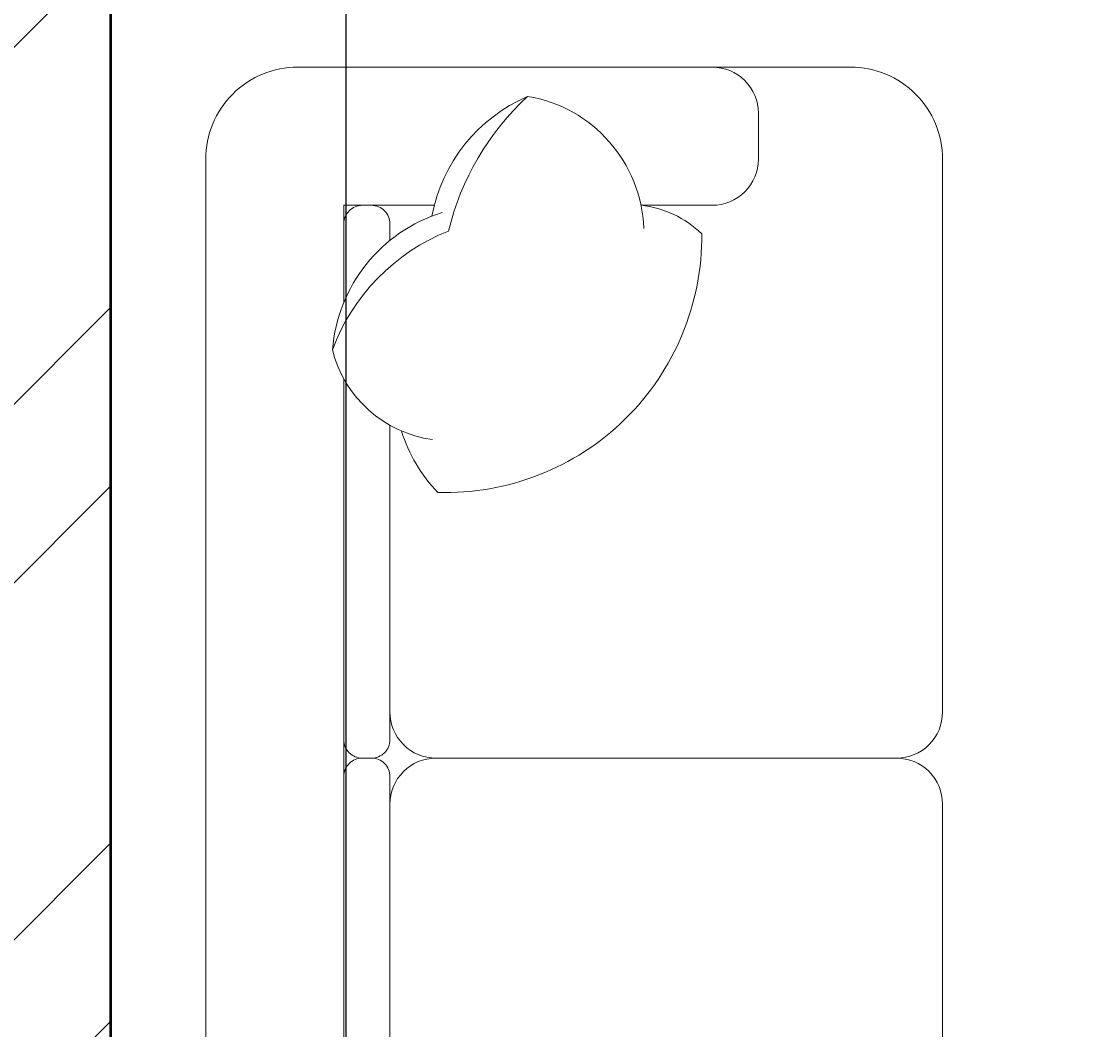
# Model space of a CAD drawing. Units: inches. Extents: x 963 to 2075, y 289 to 2657.
# Tile 51 of 98: x 1511 to 1538, y 1778 to 1803. Entities that reach past the tile are written whole.
import ezdxf

# ---------------------------------------------------------------- set-up
doc = ezdxf.new("R2010")
doc.units = ezdxf.units.IN
for name, color, linetype, lineweight in [('A-ANNO-DIMS', 2, 'Continuous', 18), ('A-FURN', 8, 'Continuous', 18), ('A-WALL', 7, 'Continuous', 50), ('A-WALL-PATT', 8, 'Continuous', 13)]:
    doc.layers.add(name, color=color, linetype=linetype, lineweight=lineweight)
doc.styles.get("Standard").update_dxf_attribs({"font": 'arial.ttf'})
doc.dimstyles.get("Standard").update_dxf_attribs({"dimtxt": 0.18, "dimasz": 0.18, "dimexe": 0.18, "dimexo": 0.0625, "dimgap": 0.09, "dimtad": 0, "dimtih": 1, "dimtoh": 1, "dimdec": 4, "dimzin": 0, "dimdsep": 46, "dimtxsty": 'Standard', "dimcen": 0.09, "dimadec": 0, "dimazin": 0, "dimtfac": 1, "dimtdec": 4, "dimtofl": 0, "dimtmove": 0, "dimatfit": 3, "dimfxl": 1, "dimtolj": 1, "dimtzin": 0, "dimarcsym": 0})

# ---------------------------------------------------------------- blocks, each defined once
blk = doc.blocks.new('*D28')
at = {"layer": 'A-ANNO-DIMS', "color": 0, "lineweight": -2, "transparency": 16777216}
for p, q in [((1506.727, 1816.319), (1519.012, 1816.319)), ((1518.832, 1816.139), (1518.832, 1775.944)), ((1518.832, 1735.382), (1518.832, 1775.577)), ((1506.727, 1735.202), (1519.012, 1735.202))]:
    blk.add_line(p, q, dxfattribs=at)
at = {"layer": 'A-ANNO-DIMS', "color": 0, "transparency": 16777216}
for points in [[(1518.802, 1816.139), (1518.862, 1816.139), (1518.832, 1816.319)], [(1518.802, 1735.382), (1518.862, 1735.382), (1518.832, 1735.202)]]:
    blk.add_solid(points, dxfattribs=at)
at = {"layer": 'Defpoints', "color": 0, "transparency": 16777216}
for p in [(1506.665, 1816.319), (1518.832, 1816.319), (1506.665, 1735.202)]:
    blk.add_point(p, dxfattribs=at)
at = {"layer": 'A-ANNO-DIMS', "color": 0, "transparency": 16777216, "insert": (1518.832, 1775.761), "char_height": 0.18, "attachment_point": 5}
blk.add_mtext('\\A1;3-SEAT SOFA 81 TYP.', dxfattribs=at)

msp = doc.modelspace()

# ---------------------------------------------------------------- hatches: boundary and pattern name
at = {"layer": 'A-WALL-PATT'}
h = msp.add_hatch(dxfattribs=at)
h.set_pattern_fill('ANSI32', color=256)
h.paths.add_polyline_path([(1473.609, 2163.068), (1473.609, 2165.318), (1376.422, 2165.318), (1376.422, 2227.983), (1371.922, 2227.983), (1371.922, 2214.818), (1368.405, 2214.818), (1368.405, 2210.318), (1371.922, 2210.318), (1371.922, 2160.818), (1395.922, 2160.818), (1395.922, 2090.318), (1217.345, 2090.318), (1217.345, 2085.818), (1395.922, 2085.818), (1458.922, 2085.818), (1458.922, 2108.318), (1454.422, 2108.318), (1454.422, 2090.318), (1400.422, 2090.318), (1400.422, 2160.818), (1473.609, 2160.818)])
h.paths.add_polyline_path([(1649.422, 2210.318), (1653.225, 2210.318), (1653.225, 2214.818), (1649.422, 2214.818), (1649.422, 2227.983), (1644.922, 2227.983), (1644.922, 2165.318), (1550.099, 2165.318), (1550.099, 2160.818), (1620.922, 2160.818), (1620.922, 2112.818), (1555.446, 2112.818), (1555.446, 2108.318), (1584.327, 2108.318), (1584.327, 2084.916), (1588.827, 2084.916), (1588.827, 2108.318), (1625.422, 2108.318), (1667.951, 2108.318), (1667.951, 2022.667), (1588.827, 2022.667), (1588.827, 2047.408), (1584.327, 2047.408), (1584.327, 1996.003), (1588.827, 1996.003), (1588.827, 2018.318), (1667.951, 2018.167), (1667.951, 1928.318), (1625.422, 1928.318), (1625.422, 1923.818), (1672.451, 1923.818), (1672.451, 1928.318), (1672.451, 1946.663), (1785.446, 1946.663), (1785.446, 1951.163), (1743.034, 1951.163), (1743.034, 2017.922), (1841.422, 2017.922), (1841.422, 2014.775), (1845.922, 2014.775), (1845.922, 2017.922), (1905.922, 2017.922), (1905.922, 1987.511), (1910.422, 1987.511), (1910.422, 2022.422), (1910.422, 2068.517), (1905.922, 2068.517), (1905.922, 2022.422), (1845.922, 2022.422), (1845.922, 2025.851), (1843.672, 2025.851), (1841.422, 2025.851), (1841.422, 2022.422), (1743.034, 2022.422), (1743.034, 2084.031), (1768.451, 2084.031), (1785.446, 2084.031), (1785.446, 2088.531), (1672.451, 2088.531), (1672.451, 2112.818), (1667.951, 2112.818), (1625.422, 2112.818), (1625.422, 2160.818), (1649.422, 2160.818)])
h.paths.add_polyline_path([(1672.451, 2084.031), (1738.534, 2084.031), (1738.534, 1951.163), (1672.451, 1951.163)], flags=16)
h.paths.add_polyline_path([(1672.451, 2084.031), (1738.534, 2084.031), (1705.492, 2017.597)], flags=0)
h.paths.add_polyline_path([(1262.766, 2085.818), (1258.266, 2085.818), (1258.266, 2023.278), (1184.422, 2023.278), (1184.422, 2018.778), (1258.266, 2018.778), (1258.266, 1950.818), (1262.766, 1950.818)])
h.paths.add_polyline_path([(1312.266, 2085.818), (1307.766, 2085.818), (1307.766, 1950.818), (1312.266, 1950.818)])
h.paths.add_polyline_path([(1458.922, 1950.818), (1395.922, 1950.818), (1216.568, 1950.818), (1216.568, 1946.318), (1346.422, 1946.318), (1395.922, 1946.318), (1395.922, 1875.818), (1371.922, 1875.818), (1371.922, 1826.318), (1368.931, 1826.318), (1368.931, 1821.818), (1371.922, 1821.818), (1371.922, 1813.622), (1376.422, 1813.622), (1376.422, 1871.318), (1474.504, 1871.318), (1474.504, 1873.568), (1474.504, 1875.818), (1400.422, 1875.818), (1400.422, 1946.318), (1454.422, 1946.318), (1454.422, 1928.318), (1458.922, 1928.318)])
h.paths.add_polyline_path([(1184.422, 2120.778), (1167.922, 2120.778), (1167.922, 2134.812), (1165.672, 2134.812), (1163.422, 2134.812), (1163.422, 2120.778), (1119.922, 2120.778), (1119.922, 2098.095), (1124.422, 2098.095), (1124.422, 2116.278), (1167.922, 2116.278), (1179.922, 2116.278), (1179.922, 2045.916), (1184.422, 2045.916), (1184.422, 2090.318), (1184.422, 2116.278)])
h.paths.add_polyline_path([(1124.422, 2018.778), (1179.922, 2018.778), (1179.922, 2016.294), (1184.422, 2016.294), (1184.422, 2023.278), (1184.422, 2026.588), (1182.172, 2026.588), (1179.922, 2026.588), (1179.922, 2023.278), (1124.422, 2023.278), (1124.422, 2074.095), (1119.922, 2074.095), (1119.922, 2018.778), (1119.922, 1979.633), (1124.422, 1979.633)])
h.paths.add_polyline_path([(1184.422, 1925.778), (1184.422, 1946.318), (1184.422, 1996.073), (1182.172, 1996.073), (1179.922, 1996.073), (1179.922, 1925.778), (1124.422, 1925.778), (1124.422, 1955.633), (1119.922, 1955.502), (1119.922, 1921.278), (1158.922, 1921.278), (1158.922, 1909.983), (1163.422, 1909.983), (1163.422, 1921.278), (1184.422, 1921.278)])
h.paths.add_polyline_path([(1341.449, 1826.318), (1163.422, 1826.318), (1163.422, 1849.983), (1158.922, 1849.983), (1158.922, 1821.818), (1158.922, 1804.033), (1163.422, 1804.033), (1163.422, 1821.818), (1341.449, 1821.818)])
h.paths.add_polyline_path([(1222.981, 1713.818), (1163.422, 1713.818), (1163.422, 1744.033), (1161.172, 1744.033), (1158.922, 1744.033), (1158.922, 1713.818), (1119.922, 1713.818), (1119.922, 1694.65), (1124.422, 1694.65), (1124.422, 1709.318), (1158.922, 1709.318), (1222.981, 1709.318)])
h.paths.add_polyline_path([(1328.422, 1713.818), (1252.042, 1713.818), (1252.042, 1711.568), (1252.042, 1709.318), (1256.422, 1709.318), (1256.422, 1547.318), (1232.937, 1547.318), (1232.937, 1545.068), (1232.937, 1542.818), (1292.422, 1542.818), (1292.422, 1527.634), (1296.922, 1527.634), (1296.922, 1542.818), (1299.464, 1542.818), (1299.464, 1547.318), (1260.922, 1547.318), (1260.922, 1658.318), (1343.661, 1658.318), (1343.661, 1660.568), (1343.661, 1662.818), (1328.422, 1662.818), (1328.422, 1676.589), (1327.402, 1676.589), (1323.922, 1676.589), (1323.922, 1662.818), (1260.922, 1662.818), (1260.922, 1709.318), (1323.922, 1709.318), (1323.922, 1699.851), (1328.422, 1699.851)])
h.paths.add_polyline_path([(1649.422, 1875.818), (1625.422, 1875.818), (1625.422, 1928.318), (1620.922, 1928.318), (1588.827, 1928.318), (1588.827, 1950.59), (1584.327, 1950.59), (1584.327, 1928.318), (1555.446, 1928.318), (1555.446, 1923.818), (1620.922, 1923.818), (1620.922, 1875.818), (1548.952, 1875.818), (1548.952, 1873.568), (1548.952, 1871.318), (1644.922, 1871.318), (1644.922, 1813.622), (1649.422, 1813.622), (1649.422, 1821.818), (1652.045, 1821.818), (1652.045, 1824.068), (1652.045, 1826.318), (1649.422, 1826.318)])
h.paths.add_polyline_path([(1512.922, 1871.318), (1516.476, 1871.318), (1516.476, 1875.818), (1512.922, 1875.818), (1512.922, 1923.818), (1512.922, 1928.318), (1512.922, 1930.827), (1508.422, 1930.827), (1508.422, 1875.818), (1504.411, 1875.818), (1504.411, 1871.318), (1508.422, 1871.318), (1508.422, 1713.818), (1376.422, 1713.818), (1376.422, 1743.325), (1371.922, 1743.325), (1371.922, 1709.318), (1371.922, 1706.01), (1376.422, 1706.01), (1376.422, 1709.318), (1508.422, 1709.318), (1508.422, 1547.318), (1501.871, 1547.318), (1501.871, 1542.818), (1508.422, 1542.818), (1508.422, 1482.818), (1508.422, 1436.318), (1512.922, 1436.318), (1512.922, 1542.818), (1519.318, 1542.818), (1519.318, 1545.068), (1519.318, 1547.318), (1512.922, 1547.318), (1512.922, 1709.318), (1644.922, 1709.318), (1644.922, 1707.548), (1649.422, 1707.548), (1649.422, 1709.318), (1649.422, 1743.325), (1644.922, 1743.325), (1644.922, 1713.818), (1512.922, 1713.818)])
h.paths.add_polyline_path([(1129.884, 1545.068), (1129.884, 1547.318), (1124.422, 1547.318), (1095.922, 1547.318), (1095.922, 1614.818), (1124.422, 1614.818), (1124.422, 1619.318), (1095.922, 1619.318), (1091.422, 1619.318), (1091.422, 1542.818), (1095.922, 1542.818), (1119.922, 1542.818), (1129.884, 1542.818)])
h.paths.add_polyline_path([(1208.422, 1542.818), (1211.74, 1542.818), (1211.74, 1547.318), (1198.851, 1547.318), (1198.851, 1542.818), (1203.922, 1542.818), (1203.922, 1478.318), (1208.422, 1478.318), (1296.922, 1478.318), (1296.922, 1503.634), (1292.422, 1503.634), (1292.422, 1482.818), (1208.422, 1482.818)])
h.paths.add_polyline_path([(1430.422, 1542.818), (1435.699, 1542.818), (1435.699, 1545.068), (1435.699, 1547.318), (1422.658, 1547.318), (1422.658, 1545.068), (1422.658, 1542.818), (1425.922, 1542.818), (1425.922, 1482.857), (1341.922, 1482.857), (1341.922, 1502.732), (1337.422, 1502.732), (1337.422, 1478.357), (1425.922, 1478.357), (1425.922, 1440.818), (1425.922, 1436.318), (1430.422, 1436.318)])
h.paths.add_polyline_path([(1698.482, 2004.259), (1727.695, 2004.259), (1727.695, 2022.916), (1698.482, 2022.916)], flags=8)

# ---------------------------------------------------------------- linework, layer by layer
at = {"layer": 'A-FURN', "ltscale": 0.03}
msp.add_lwpolyline([(1531.529, 1801.839, -0.414214), (1533.846, 1799.522), (1533.846, 1785.616, -0.414214), (1532.687, 1784.457, -0.414214), (1533.846, 1783.298), (1533.846, 1771.71, -0.414214), (1532.687, 1770.552, -0.414214), (1533.846, 1769.393), (1533.846, 1755.487, -0.414214), (1531.529, 1753.169), (1517.623, 1753.169, -0.414214), (1515.305, 1755.487), (1515.305, 1799.522, -0.414214), (1517.623, 1801.839)], format="xyb", close=True, dxfattribs=at)
at = {"layer": 'A-FURN'}
for points in [[(1528.052, 1801.839, -0.414214), (1529.211, 1800.68), (1529.211, 1799.522, -0.414214), (1528.052, 1798.363), (1526.257, 1798.363)], [(1523.406, 1801.102, 0.14773), (1521.415, 1797.715, 0.213343), (1518.494, 1794.727, 0.178662)], [(1526.327, 1797.781, 0.356772), (1523.406, 1801.102, 0.249542), (1520.999, 1798.093, -9.61688)], [(1519.941, 1797.479), (1519.941, 1797.899, 0.414214), (1519.477, 1798.363), (1519.245, 1798.363, 0.414214), (1518.782, 1797.899)], [(1526.256, 1798.365, -0.165541), (1527.787, 1797.649, -0.425989), (1521.149, 1791.14, -0.121523), (1520.234, 1792.685, 7.115464)], [(1521.256, 1798.183, 0.306663), (1518.494, 1794.727, 0.30633), (1521.016, 1792.469, -0.872847)], [(1518.782, 1797.899), (1518.782, 1795.925, 0.414214)], [(1518.782, 1793.997), (1518.782, 1784.921, 0.414214), (1519.245, 1784.457), (1519.477, 1784.457, 0.414214), (1519.941, 1784.921), (1519.941, 1792.83, 0.414214)], [(1519.941, 1785.616, 0.414214), (1521.099, 1784.457), (1532.687, 1784.457, 0.414214)], [(1519.941, 1783.298, -0.414214), (1521.099, 1784.457)]]:
    msp.add_lwpolyline(points, format="xyb", dxfattribs=at)
for points in [[(1521.059, 1798.363), (1518.782, 1798.363), (1518.782, 1795.925)], [(1518.782, 1793.997), (1518.782, 1767.254)]]:
    msp.add_lwpolyline(points, dxfattribs=at)
msp.add_lwpolyline([(1518.782, 1771.015), (1518.782, 1783.994, -0.414214), (1519.245, 1784.457), (1519.477, 1784.457, -0.414214), (1519.941, 1783.994), (1519.941, 1771.015, -0.414214), (1519.477, 1770.552), (1519.245, 1770.552, -0.414214)], format="xyb", close=True, dxfattribs=at)
at = {"layer": 'A-WALL'}
msp.add_line((1512.922, 1713.818), (1512.922, 1871.318), dxfattribs=at)

# ---------------------------------------------------------------- dimensions: what is measured, and where the dimension line sits
at = {"layer": 'A-ANNO-DIMS'}
dim = msp.add_linear_dim(base=(1518.832, 1816.319), p1=(1506.665, 1735.202), p2=(1506.665, 1816.319), angle=90, text='3-SEAT SOFA <> TYP.', dimstyle='Standard', override={"dimdec": 0, "dimlfac": 1, "dimrnd": 0, "dimzin": 0, "dimdsep": 46, "dimlunit": 2}, dxfattribs=at)
dim.commit()
dim.dimension.update_dxf_attribs({"geometry": '*D28', "text_midpoint": (1518.832, 1775.761)})

doc.saveas('drawing.dxf')
